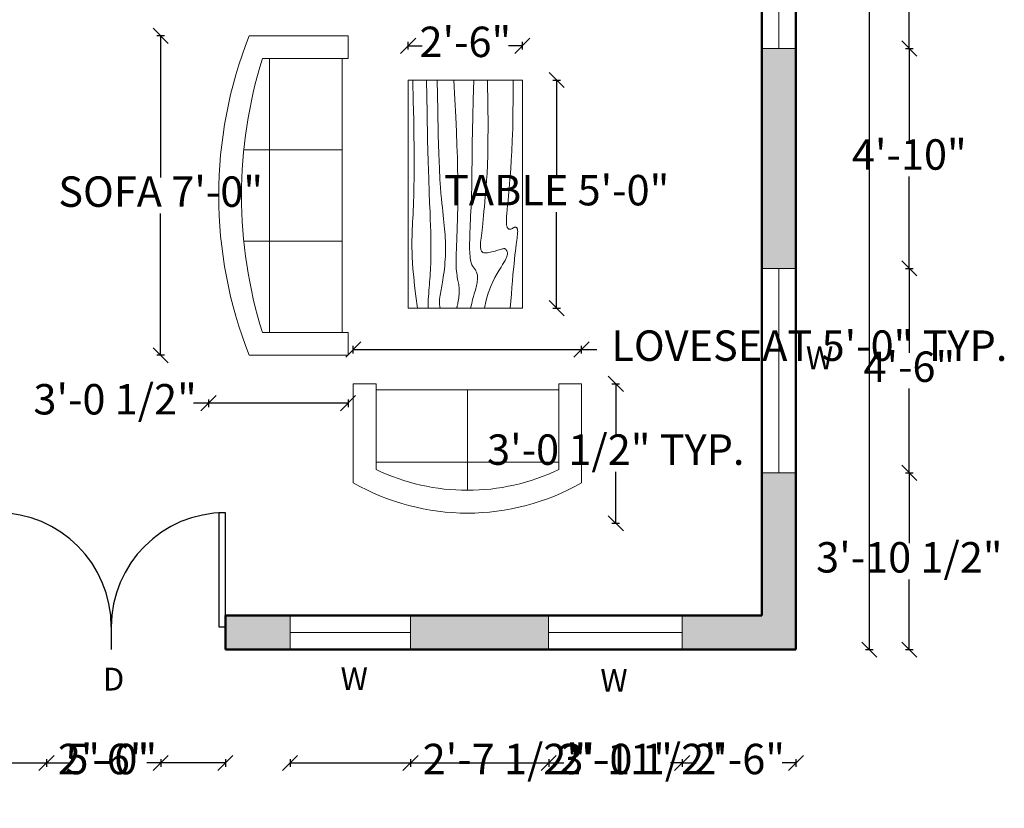
# Model space of a CAD drawing. Units: inches. Extents: x 2395 to 2921, y 528 to 1164.
# Tile 3 of 5: x 2662 to 2921, y 528 to 735. Entities that reach past the tile are written whole.
import ezdxf

# ---------------------------------------------------------------- set-up
doc = ezdxf.new("R2010")
doc.units = ezdxf.units.IN
for name, color, linetype, lineweight in [('A-ANNO-DIMS', 2, 'Continuous', 18), ('A-ANNO-TEXT', 7, 'Continuous', 18), ('A-DOOR', 3, 'Continuous', 25), ('A-FURN', 8, 'Continuous', 18), ('A-GLAZ', 4, 'Continuous', 18), ('A-WALL', 162, 'Continuous', 50), ('A-WALL-PATT', 162, 'Continuous', 13)]:
    doc.layers.add(name, color=color, linetype=linetype, lineweight=lineweight)
doc.styles.get("Standard").update_dxf_attribs({"font": 'arial.ttf'})
doc.dimstyles.new('ISO-25', dxfattribs={"dimtxt": 8, "dimasz": 4, "dimexe": 1, "dimexo": 1, "dimtad": 0, "dimtih": 1, "dimtoh": 1, "dimlunit": 3, "dimtxsty": 'Standard', "dimblk": 'OBLIQUE', "dimcen": 2.5, "dimadec": 0, "dimazin": 0, "dimtfac": 1, "dimtmove": 0, "dimatfit": 3, "dimfxl": 1, "dimfxlon": 1, "dimarcsym": 0})

# ---------------------------------------------------------------- blocks, each defined once
blk = doc.blocks.new('*U4')
for p, q in [((-30, 0), (-30, -6)), ((0, 0), (0, -6))]:
    blk.add_line(p, q)
blk.add_lwpolyline([(0, 0), (0, 30), (-1.75, 30), (-1.75, 0)], close=True)
blk.add_arc((0, 0), 30, 90, 180)
blk = doc.blocks.new('*U6')
for p, q in [((0, 0), (0, -6)), ((30, 0), (30, -6))]:
    blk.add_line(p, q)
blk.add_lwpolyline([(0, 0), (0, 30), (1.75, 30), (1.75, 0)], close=True)
blk.add_arc((0, 0), 30, 0, 90)
blk = doc.blocks.new('Sofa - Roundback 7 ft.')
for p, q in [((-12.00002, -32.4421), (-12.00003, -6.5971)), ((11.99997, -32.4421), (11.99998, -6.5971)), ((-36.000027, -34), (-36.000027, -11.4696)), ((35.99998, -34), (35.99998, -11.4696)), ((-35.999844, -13.3819), (35.9998, -13.3819)), ((-36.000027, -32.4421), (35.99998, -32.4421))]:
    blk.add_line(p, q)
for points in [[(-36.000027, -34), (-42.000027, -34), (-42.000027, -8)], [(41.99998, -8), (41.99998, -34), (35.99998, -34)]]:
    blk.add_lwpolyline(points)
for centre, radius, start, end in [((0, -114.25), 114.25, 68.43141, 111.5686), ((-0.00001, -127.1968), 121.1968, 72.72033, 107.2797)]:
    blk.add_arc(centre, radius, start, end)
blk = doc.blocks.new('Table - Rectangular Woodgrain 60 x 30 in.')
for p, q in [((0, 0), (0, -30)), ((60, 0), (0, 0)), ((60, -30), (60, 0)), ((0, -30), (60, -30))]:
    blk.add_line(p, q)
for points in [[(0, -2.4), (4.8155, -2.418), (9.0302, -2.4688), (12.709, -2.5477), (15.9167, -2.65), (18.7181, -2.7711), (21.1781, -2.9063), (23.3616, -3.0508), (25.3333, -3.2), (27.1477, -3.3495), (28.8172, -3.4958), (30.3437, -3.636), (31.7291, -3.7667), (32.9756, -3.8849), (34.0849, -3.9875), (35.059, -4.0714), (35.9, -4.1334), (36.6114, -4.1711), (37.2041, -4.1854), (37.6906, -4.1779), (38.0833, -4.15), (38.3948, -4.1034), (38.6375, -4.0396), (38.8239, -3.9602), (38.9666, -3.8667), (39.0764, -3.7608), (39.1573, -3.6448), (39.2116, -3.521), (39.2416, -3.3917), (39.2498, -3.2593), (39.2385, -3.1261), (39.21, -2.9944), (39.1666, -2.8667), (39.111, -2.7447), (39.0468, -2.6281), (38.978, -2.5163), (38.9083, -2.4083), (38.8418, -2.3035), (38.7823, -2.201), (38.7337, -2.1001), (38.7, -2), (38.6844, -1.9003), (38.6875, -1.8021), (38.7094, -1.707), (38.75, -1.6167), (38.8094, -1.5326), (38.8875, -1.4563), (38.9844, -1.3893), (39.1, -1.3333), (39.2351, -1.2896), (39.3937, -1.2583), (39.5804, -1.2396), (39.8, -1.2333), (40.057, -1.2396), (40.3562, -1.2583), (40.7023, -1.2896), (41.1, -1.3333), (41.5547, -1.3895), (42.0755, -1.4573), (42.6721, -1.5361), (43.3542, -1.625), (44.1316, -1.7233), (45.014, -1.8302), (46.0114, -1.9449), (47.1333, -2.0667), (48.3862, -2.1947), (49.7625, -2.3281), (51.2513, -2.4663), (52.8416, -2.6083), (54.5226, -2.7535), (56.2833, -2.9011), (58.1127, -3.0501), (60, -3.2)], [(0, -9.2), (6.5759, -9.0858), (11.9385, -9.0365), (16.2527, -9.0418), (19.6833, -9.0917), (22.3952, -9.1759), (24.5531, -9.2844), (26.322, -9.4069), (27.8666, -9.5333), (29.3241, -9.6553), (30.7203, -9.7719), (32.0532, -9.8837), (33.3208, -9.9917), (34.5213, -10.0965), (35.6526, -10.199), (36.7128, -10.2999), (37.7, -10.4), (38.6129, -10.4996), (39.4531, -10.5969), (40.223, -10.6895), (40.925, -10.775), (41.5613, -10.8512), (42.1344, -10.9156), (42.6465, -10.966), (43.1, -11), (43.4976, -11.0158), (43.8437, -11.0136), (44.143, -10.9942), (44.4, -10.9583), (44.6195, -10.9069), (44.8062, -10.8406), (44.9648, -10.7603), (45.1, -10.6667), (45.2155, -10.5598), (45.3114, -10.4365), (45.3871, -10.2929), (45.4416, -10.125), (45.4743, -9.929), (45.4844, -9.7011), (45.4709, -9.4371), (45.4333, -9.1333), (45.3716, -8.7883), (45.2896, -8.4104), (45.1919, -8.0107), (45.0833, -7.6), (44.9685, -7.1893), (44.8521, -6.7896), (44.7388, -6.4117), (44.6333, -6.0667), (44.54, -5.7628), (44.4614, -5.4979), (44.4001, -5.2675), (44.3583, -5.0667), (44.3384, -4.8909), (44.3427, -4.7354), (44.3736, -4.5956), (44.4333, -4.4667), (44.5236, -4.3453), (44.6427, -4.2333), (44.7884, -4.1339), (44.9583, -4.05), (45.1501, -3.9849), (45.3614, -3.9417), (45.59, -3.9234), (45.8333, -3.9333), (46.0915, -3.9749), (46.3734, -4.0531), (46.6906, -4.1736), (47.0542, -4.3417), (47.4756, -4.5629), (47.9661, -4.8427), (48.5372, -5.1866), (49.2, -5.6), (49.9676, -6.0844), (50.8594, -6.625), (51.8965, -7.2031), (53.1, -7.8), (54.491, -8.3969), (56.0906, -8.975), (57.9199, -9.5156), (60, -10)], [(0, -12.8), (5.1847, -12.9322), (9.6213, -13.0323), (13.3963, -13.1059), (16.5958, -13.1583), (19.3063, -13.1952), (21.614, -13.2219), (23.6054, -13.2439), (25.3666, -13.2667), (26.9728, -13.2947), (28.4531, -13.3281), (29.8256, -13.3663), (31.1083, -13.4083), (32.3191, -13.4535), (33.476, -13.501), (34.597, -13.5501), (35.7, -13.6), (36.7984, -13.6497), (37.8875, -13.6979), (38.9578, -13.743), (40, -13.7833), (41.0047, -13.8174), (41.9625, -13.8438), (42.864, -13.8607), (43.7, -13.8667), (44.4631, -13.8604), (45.1552, -13.8417), (45.7801, -13.8104), (46.3416, -13.7667), (46.8439, -13.7104), (47.2906, -13.6417), (47.6858, -13.5604), (48.0333, -13.4667), (48.3375, -13.3608), (48.6042, -13.2448), (48.8396, -13.121), (49.05, -12.9917), (49.2417, -12.8593), (49.4208, -12.7261), (49.5937, -12.5944), (49.7667, -12.4667), (49.9452, -12.3451), (50.1323, -12.2313), (50.3303, -12.1268), (50.5416, -12.0333), (50.7686, -11.9524), (51.0135, -11.8854), (51.2788, -11.8341), (51.5666, -11.8), (51.8785, -11.7843), (52.2116, -11.7865), (52.562, -11.8059), (52.926, -11.8417), (53.2998, -11.8931), (53.6795, -11.9594), (54.0614, -12.0397), (54.4416, -12.1333), (54.8223, -12.2401), (55.2293, -12.3625), (55.6942, -12.5037), (56.2489, -12.6667), (56.9251, -12.8547), (57.7545, -13.0708), (58.7689, -13.3182), (60, -13.6)], [(0, -18), (5.124, -17.7273), (9.6609, -17.5057), (13.6705, -17.3303), (17.2125, -17.1958), (20.3467, -17.0973), (23.1328, -17.0297), (25.6307, -16.9878), (27.9, -16.9667), (29.9928, -16.9617), (31.9302, -16.9703), (33.7254, -16.9907), (35.3917, -17.0208), (36.9423, -17.0588), (38.3906, -17.1026), (39.7499, -17.1503), (41.0333, -17.2), (42.2519, -17.2496), (43.4073, -17.2969), (44.4986, -17.3395), (45.525, -17.375), (46.4858, -17.4012), (47.3802, -17.4156), (48.2074, -17.416), (48.9667, -17.4), (49.6583, -17.3662), (50.2872, -17.3167), (50.8595, -17.2547), (51.3812, -17.1833), (51.8584, -17.1057), (52.2971, -17.025), (52.7034, -16.9443), (53.0833, -16.8667), (53.443, -16.7951), (53.789, -16.7313), (54.128, -16.6768), (54.4666, -16.6334), (54.8115, -16.6024), (55.1693, -16.5854), (55.5465, -16.5841), (55.95, -16.6), (56.3828, -16.6337), (56.8346, -16.6823), (57.2915, -16.7418), (57.7396, -16.8084), (58.165, -16.878), (58.5539, -16.9469), (58.8924, -17.0111), (59.1666, -17.0667), (59.3679, -17.1107), (59.5078, -17.1438), (59.6032, -17.1675), (59.6708, -17.1833), (59.7275, -17.193), (59.7901, -17.1979), (59.8753, -17.1998), (60, -17.2)], [(0, -22.4), (8.0098, -22.2501), (14.4094, -22.1011), (19.4168, -21.9535), (23.25, -21.8083), (26.1269, -21.6663), (28.2656, -21.5281), (29.884, -21.3947), (31.2, -21.2667), (32.3967, -21.1448), (33.5172, -21.0292), (34.5697, -20.9198), (35.5625, -20.8167), (36.5037, -20.7198), (37.4015, -20.6292), (38.2642, -20.5448), (39.1, -20.4667), (39.9164, -20.3951), (40.7187, -20.3313), (41.5117, -20.2768), (42.3, -20.2333), (43.0883, -20.2024), (43.8812, -20.1854), (44.6836, -20.1841), (45.5, -20.2), (46.3328, -20.234), (47.1747, -20.2844), (48.0163, -20.3488), (48.8479, -20.425), (49.66, -20.5106), (50.4429, -20.6031), (51.1872, -20.7004), (51.8833, -20.8), (52.5246, -20.8999), (53.1166, -20.9995), (53.6681, -21.0983), (54.1875, -21.1958), (54.6834, -21.2919), (55.1646, -21.3859), (55.6394, -21.4777), (56.1167, -21.5667), (56.6028, -21.6515), (57.0961, -21.7266), (57.5929, -21.7852), (58.0896, -21.8208), (58.5823, -21.8268), (59.0674, -21.7964), (59.5412, -21.723), (60, -21.6)], [(0, -25.2), (8.6355, -25.0504), (15.7026, -24.9031), (21.4049, -24.7606), (25.9458, -24.625), (29.529, -24.4988), (32.3578, -24.3844), (34.6359, -24.284), (36.5667, -24.2), (38.3213, -24.1341), (39.9417, -24.0854), (41.437, -24.0523), (42.8167, -24.0333), (44.0901, -24.0268), (45.2667, -24.0313), (46.3557, -24.0451), (47.3667, -24.0667), (48.309, -24.0947), (49.1928, -24.1287), (50.0284, -24.168), (50.826, -24.2125), (51.5959, -24.2617), (52.3483, -24.3151), (53.0935, -24.3725), (53.8417, -24.4334), (54.6009, -24.497), (55.3699, -24.561), (56.1454, -24.6226), (56.9239, -24.6792), (57.7021, -24.7279), (58.4764, -24.7662), (59.2435, -24.7911), (60, -24.8)], [(0, -28.8), (5.6867, -28.6681), (10.45, -28.5698), (14.407, -28.5012), (17.675, -28.4584), (20.3711, -28.4374), (22.6125, -28.4344), (24.5164, -28.4455), (26.2, -28.4667), (27.762, -28.4947), (29.2276, -28.5281), (30.6033, -28.5663), (31.8958, -28.6084), (33.1118, -28.6535), (34.2578, -28.7011), (35.3405, -28.7501), (36.3666, -28.8), (37.3443, -28.8497), (38.288, -28.8974), (39.2137, -28.9412), (40.1375, -28.9792), (41.0753, -29.0093), (42.0432, -29.0297), (43.0572, -29.0384), (44.1333, -29.0333), (45.2936, -29.0114), (46.5843, -28.9641), (48.0579, -28.8816), (49.7666, -28.7542), (51.7629, -28.5721), (54.0989, -28.3255), (56.8272, -28.0048), (60, -27.6)]]:
    blk.add_lwpolyline(points)
blk = doc.blocks.new('Sofa - Roundback Loveseat 5 ft.')
for p, q in [((0, -32.44198), (0, -5.99998)), ((-24, -33.99998), (-24, -11.46958)), ((24.00004, -33.99998), (24.00004, -11.46958)), ((-23.9998, -13.38178), (23.99986, -13.38178)), ((-24, -32.44198), (24.00004, -32.44198))]:
    blk.add_line(p, q)
for points in [[(-24, -33.99998), (-30, -33.99998), (-30, -7.99998)], [(30.00004, -7.99998), (30.00004, -33.99998), (24.00004, -33.99998)]]:
    blk.add_lwpolyline(points)
for centre, radius, start, end in [((0, -60.24998), 60.24998, 60.13715, 119.8628), ((0, -61.38438), 55.38444, 64.32083, 115.6792)]:
    blk.add_arc(centre, radius, start, end)
blk = doc.blocks.new('_Oblique')
at = {"color": 0, "linetype": 'ByBlock', "lineweight": -2}
blk.add_line((-0.5, -0.5), (0.5, 0.5), dxfattribs=at)
blk = doc.blocks.new('*D20')
at = {"layer": 'A-ANNO-DIMS', "color": 0, "lineweight": -2, "transparency": 16777216}
for p, q in [((2884.49, 1121.85), (2886.49, 1121.85)), ((2885.49, 1121.85), (2885.49, 850.56)), ((2885.49, 569.85), (2885.49, 841.14)), ((2884.49, 569.85), (2886.49, 569.85))]:
    blk.add_line(p, q, dxfattribs=at)
at = {"layer": 'Defpoints', "color": 0, "transparency": 16777216}
for p in [(2866.2, 1121.85), (2866.2, 569.85), (2885.49, 569.85)]:
    blk.add_point(p, dxfattribs=at)
at = {"layer": 'A-ANNO-DIMS', "color": 0, "lineweight": -2, "transparency": 16777216, "xscale": 4, "yscale": 4, "zscale": 4}
for p, rotation in [((2885.49, 1121.85), 90), ((2885.49, 569.85), 270)]:
    blk.add_blockref('_Oblique', p, dxfattribs=dict(at, rotation=rotation))
at = {"layer": 'A-ANNO-DIMS', "color": 0, "transparency": 16777216, "insert": (2885.49, 845.85), "char_height": 8, "attachment_point": 5}
blk.add_mtext("46'", dxfattribs=at)
blk = doc.blocks.new('*D28')
at = {"layer": 'A-ANNO-DIMS', "color": 0, "lineweight": -2, "transparency": 16777216}
for p, q in [((2749.83, 647.74), (2749.83, 649.74)), ((2809.83, 647.74), (2809.83, 649.74)), ((2749.83, 648.74), (2809.83, 648.74)), ((2809.83, 648.74), (2813.83, 648.74))]:
    blk.add_line(p, q, dxfattribs=at)
at = {"layer": 'Defpoints', "color": 0, "transparency": 16777216}
for p in [(2809.83, 648.74), (2749.83, 639.74), (2809.83, 639.74)]:
    blk.add_point(p, dxfattribs=at)
at = {"layer": 'A-ANNO-DIMS', "color": 0, "lineweight": -2, "transparency": 16777216, "xscale": 4, "yscale": 4, "zscale": 4, "rotation": 180}
blk.add_blockref('_Oblique', (2749.83, 648.74), dxfattribs=at)
at = {"layer": 'A-ANNO-DIMS', "color": 0, "lineweight": -2, "transparency": 16777216, "xscale": 4, "yscale": 4, "zscale": 4}
blk.add_blockref('_Oblique', (2809.83, 648.74), dxfattribs=at)
at = {"layer": 'A-ANNO-DIMS', "color": 0, "transparency": 16777216, "insert": (2869.72, 648.74), "char_height": 8, "attachment_point": 5}
blk.add_mtext('LOVESEAT 5\'-0" TYP.', dxfattribs=at)
blk = doc.blocks.new('*D29')
at = {"layer": 'A-ANNO-DIMS', "color": 0, "lineweight": -2, "transparency": 16777216}
for p, q in [((2817.83, 639.74), (2819.83, 639.74)), ((2818.83, 639.74), (2818.83, 626.17)), ((2818.83, 603.07), (2818.83, 616.64)), ((2817.83, 603.07), (2819.83, 603.07))]:
    blk.add_line(p, q, dxfattribs=at)
at = {"layer": 'Defpoints', "color": 0, "transparency": 16777216}
for p in [(2809.83, 639.74), (2809.83, 603.07), (2818.83, 603.07)]:
    blk.add_point(p, dxfattribs=at)
at = {"layer": 'A-ANNO-DIMS', "color": 0, "lineweight": -2, "transparency": 16777216, "xscale": 4, "yscale": 4, "zscale": 4}
for p, rotation in [((2818.83, 639.74), 90), ((2818.83, 603.07), 270)]:
    blk.add_blockref('_Oblique', p, dxfattribs=dict(at, rotation=rotation))
at = {"layer": 'A-ANNO-DIMS', "color": 0, "transparency": 16777216, "insert": (2818.83, 621.4), "char_height": 8, "attachment_point": 5}
blk.add_mtext('3\'-0 1/2" TYP.', dxfattribs=at)
blk = doc.blocks.new('*D32')
at = {"layer": 'A-ANNO-DIMS', "color": 0, "lineweight": -2, "transparency": 16777216}
for p, q in [((2700.18, 731.24), (2698.18, 731.24)), ((2699.18, 731.24), (2699.18, 694.01)), ((2699.18, 647.24), (2699.18, 684.48)), ((2700.18, 647.24), (2698.18, 647.24))]:
    blk.add_line(p, q, dxfattribs=at)
at = {"layer": 'Defpoints', "color": 0, "transparency": 16777216}
for p in [(2699.18, 731.24), (2711.78, 731.24), (2711.78, 647.24)]:
    blk.add_point(p, dxfattribs=at)
at = {"layer": 'A-ANNO-DIMS', "color": 0, "lineweight": -2, "transparency": 16777216, "xscale": 4, "yscale": 4, "zscale": 4}
for p, rotation in [((2699.18, 731.24), 90), ((2699.18, 647.24), 270)]:
    blk.add_blockref('_Oblique', p, dxfattribs=dict(at, rotation=rotation))
at = {"layer": 'A-ANNO-DIMS', "color": 0, "transparency": 16777216, "insert": (2699.18, 689.24), "char_height": 8, "attachment_point": 5}
blk.add_mtext('SOFA 7\'-0"', dxfattribs=at)
blk = doc.blocks.new('*D33')
at = {"layer": 'A-ANNO-DIMS', "color": 0, "lineweight": -2, "transparency": 16777216}
for p, q in [((2711.78, 634.64), (2707.78, 634.64)), ((2711.78, 635.64), (2711.78, 633.64)), ((2748.45, 634.64), (2711.78, 634.64)), ((2748.45, 635.64), (2748.45, 633.64))]:
    blk.add_line(p, q, dxfattribs=at)
at = {"layer": 'Defpoints', "color": 0, "transparency": 16777216}
for p in [(2711.78, 647.24), (2748.45, 647.24), (2711.78, 634.64)]:
    blk.add_point(p, dxfattribs=at)
at = {"layer": 'A-ANNO-DIMS', "color": 0, "lineweight": -2, "transparency": 16777216, "xscale": 4, "yscale": 4, "zscale": 4, "rotation": 180}
blk.add_blockref('_Oblique', (2711.78, 634.64), dxfattribs=at)
at = {"layer": 'A-ANNO-DIMS', "color": 0, "lineweight": -2, "transparency": 16777216, "xscale": 4, "yscale": 4, "zscale": 4}
blk.add_blockref('_Oblique', (2748.45, 634.64), dxfattribs=at)
at = {"layer": 'A-ANNO-DIMS', "color": 0, "transparency": 16777216, "insert": (2687.21, 634.64), "char_height": 8, "attachment_point": 5}
blk.add_mtext('3\'-0 1/2"', dxfattribs=at)
blk = doc.blocks.new('*D34')
at = {"layer": 'A-ANNO-DIMS', "color": 0, "lineweight": -2, "transparency": 16777216}
for p, q in [((2802.28, 719.62), (2804.28, 719.62)), ((2803.28, 719.62), (2803.28, 694.33)), ((2803.28, 659.62), (2803.28, 684.91)), ((2802.28, 659.62), (2804.28, 659.62))]:
    blk.add_line(p, q, dxfattribs=at)
at = {"layer": 'Defpoints', "color": 0, "transparency": 16777216}
for p in [(2794.28, 719.62), (2794.28, 659.62), (2803.28, 659.62)]:
    blk.add_point(p, dxfattribs=at)
at = {"layer": 'A-ANNO-DIMS', "color": 0, "lineweight": -2, "transparency": 16777216, "xscale": 4, "yscale": 4, "zscale": 4}
for p, rotation in [((2803.28, 719.62), 90), ((2803.28, 659.62), 270)]:
    blk.add_blockref('_Oblique', p, dxfattribs=dict(at, rotation=rotation))
at = {"layer": 'A-ANNO-DIMS', "color": 0, "transparency": 16777216, "insert": (2803.28, 689.62), "char_height": 8, "attachment_point": 5}
blk.add_mtext('TABLE 5\'-0"', dxfattribs=at)
blk = doc.blocks.new('*D35')
at = {"layer": 'A-ANNO-DIMS', "color": 0, "lineweight": -2, "transparency": 16777216}
for p, q in [((2764.28, 727.62), (2764.28, 729.62)), ((2764.28, 728.62), (2767.95, 728.62)), ((2794.28, 728.62), (2790.6, 728.62)), ((2794.28, 727.62), (2794.28, 729.62))]:
    blk.add_line(p, q, dxfattribs=at)
at = {"layer": 'Defpoints', "color": 0, "transparency": 16777216}
for p in [(2794.28, 728.62), (2764.28, 719.62), (2794.28, 719.62)]:
    blk.add_point(p, dxfattribs=at)
at = {"layer": 'A-ANNO-DIMS', "color": 0, "lineweight": -2, "transparency": 16777216, "xscale": 4, "yscale": 4, "zscale": 4, "rotation": 180}
blk.add_blockref('_Oblique', (2764.28, 728.62), dxfattribs=at)
at = {"layer": 'A-ANNO-DIMS', "color": 0, "lineweight": -2, "transparency": 16777216, "xscale": 4, "yscale": 4, "zscale": 4}
blk.add_blockref('_Oblique', (2794.28, 728.62), dxfattribs=at)
at = {"layer": 'A-ANNO-DIMS', "color": 0, "transparency": 16777216, "insert": (2779.28, 728.62), "char_height": 8, "attachment_point": 5}
blk.add_mtext('2\'-6"', dxfattribs=at)
blk = doc.blocks.new('*D45')
at = {"layer": 'A-ANNO-DIMS', "color": 0, "lineweight": -2, "transparency": 16777216}
for p, q in [((2656.2, 541.05), (2656.2, 539.05)), ((2716.2, 541.05), (2716.2, 539.05)), ((2656.2, 540.05), (2674.94, 540.05)), ((2716.2, 540.05), (2697.46, 540.05))]:
    blk.add_line(p, q, dxfattribs=at)
at = {"layer": 'Defpoints', "color": 0, "transparency": 16777216}
for p in [(2656.2, 569.85), (2716.2, 569.85), (2716.2, 540.05)]:
    blk.add_point(p, dxfattribs=at)
at = {"layer": 'A-ANNO-DIMS', "color": 0, "lineweight": -2, "transparency": 16777216, "xscale": 4, "yscale": 4, "zscale": 4, "rotation": 180}
blk.add_blockref('_Oblique', (2656.2, 540.05), dxfattribs=at)
at = {"layer": 'A-ANNO-DIMS', "color": 0, "lineweight": -2, "transparency": 16777216, "xscale": 4, "yscale": 4, "zscale": 4}
blk.add_blockref('_Oblique', (2716.2, 540.05), dxfattribs=at)
at = {"layer": 'A-ANNO-DIMS', "color": 0, "transparency": 16777216, "insert": (2686.2, 540.05), "char_height": 8, "attachment_point": 5}
blk.add_mtext('5\'-0"', dxfattribs=at)
blk = doc.blocks.new('*D46')
at = {"layer": 'A-ANNO-DIMS', "color": 0, "lineweight": -2, "transparency": 16777216}
for p, q in [((2733.2, 541.05), (2733.2, 539.05)), ((2764.89, 541.05), (2764.89, 539.05)), ((2733.2, 540.05), (2764.89, 540.05)), ((2764.89, 540.05), (2768.89, 540.05))]:
    blk.add_line(p, q, dxfattribs=at)
at = {"layer": 'Defpoints', "color": 0, "transparency": 16777216}
for p in [(2733.2, 569.85), (2764.89, 569.85), (2764.89, 540.05)]:
    blk.add_point(p, dxfattribs=at)
at = {"layer": 'A-ANNO-DIMS', "color": 0, "lineweight": -2, "transparency": 16777216, "xscale": 4, "yscale": 4, "zscale": 4, "rotation": 180}
blk.add_blockref('_Oblique', (2733.2, 540.05), dxfattribs=at)
at = {"layer": 'A-ANNO-DIMS', "color": 0, "lineweight": -2, "transparency": 16777216, "xscale": 4, "yscale": 4, "zscale": 4}
blk.add_blockref('_Oblique', (2764.89, 540.05), dxfattribs=at)
at = {"layer": 'A-ANNO-DIMS', "color": 0, "transparency": 16777216, "insert": (2789.54, 540.05), "char_height": 8, "attachment_point": 5}
blk.add_mtext('2\'-7 1/2"', dxfattribs=at)
blk = doc.blocks.new('*D47')
at = {"layer": 'A-ANNO-DIMS', "color": 0, "lineweight": -2, "transparency": 16777216}
for p, q in [((2764.89, 541.05), (2764.89, 539.05)), ((2801.19, 541.05), (2801.19, 539.05)), ((2764.89, 540.05), (2801.19, 540.05)), ((2801.19, 540.05), (2805.19, 540.05))]:
    blk.add_line(p, q, dxfattribs=at)
at = {"layer": 'Defpoints', "color": 0, "transparency": 16777216}
for p in [(2764.89, 569.85), (2801.19, 569.85), (2801.19, 540.05)]:
    blk.add_point(p, dxfattribs=at)
at = {"layer": 'A-ANNO-DIMS', "color": 0, "lineweight": -2, "transparency": 16777216, "xscale": 4, "yscale": 4, "zscale": 4, "rotation": 180}
blk.add_blockref('_Oblique', (2764.89, 540.05), dxfattribs=at)
at = {"layer": 'A-ANNO-DIMS', "color": 0, "lineweight": -2, "transparency": 16777216, "xscale": 4, "yscale": 4, "zscale": 4}
blk.add_blockref('_Oblique', (2801.19, 540.05), dxfattribs=at)
at = {"layer": 'A-ANNO-DIMS', "color": 0, "transparency": 16777216, "insert": (2825.76, 540.05), "char_height": 8, "attachment_point": 5}
blk.add_mtext('3\'-0 1/2"', dxfattribs=at)
blk = doc.blocks.new('*D48')
at = {"layer": 'A-ANNO-DIMS', "color": 0, "lineweight": -2, "transparency": 16777216}
for p, q in [((2801.19, 541.05), (2801.19, 539.05)), ((2836.31, 541.05), (2836.31, 539.05)), ((2801.19, 540.05), (2804.32, 540.05)), ((2836.31, 540.05), (2833.19, 540.05))]:
    blk.add_line(p, q, dxfattribs=at)
at = {"layer": 'Defpoints', "color": 0, "transparency": 16777216}
for p in [(2801.19, 569.85), (2836.31, 569.85), (2836.31, 540.05)]:
    blk.add_point(p, dxfattribs=at)
at = {"layer": 'A-ANNO-DIMS', "color": 0, "lineweight": -2, "transparency": 16777216, "xscale": 4, "yscale": 4, "zscale": 4, "rotation": 180}
blk.add_blockref('_Oblique', (2801.19, 540.05), dxfattribs=at)
at = {"layer": 'A-ANNO-DIMS', "color": 0, "lineweight": -2, "transparency": 16777216, "xscale": 4, "yscale": 4, "zscale": 4}
blk.add_blockref('_Oblique', (2836.31, 540.05), dxfattribs=at)
at = {"layer": 'A-ANNO-DIMS', "color": 0, "transparency": 16777216, "insert": (2818.75, 540.05), "char_height": 8, "attachment_point": 5}
blk.add_mtext('2\'-11"', dxfattribs=at)
blk = doc.blocks.new('*D49')
at = {"layer": 'A-ANNO-DIMS', "color": 0, "lineweight": -2, "transparency": 16777216}
for p, q in [((2836.31, 541.05), (2836.31, 539.05)), ((2866.2, 541.05), (2866.2, 539.05)), ((2836.31, 540.05), (2839.93, 540.05)), ((2866.2, 540.05), (2862.58, 540.05))]:
    blk.add_line(p, q, dxfattribs=at)
at = {"layer": 'Defpoints', "color": 0, "transparency": 16777216}
for p in [(2836.31, 569.85), (2866.2, 569.85), (2866.2, 540.05)]:
    blk.add_point(p, dxfattribs=at)
at = {"layer": 'A-ANNO-DIMS', "color": 0, "lineweight": -2, "transparency": 16777216, "xscale": 4, "yscale": 4, "zscale": 4, "rotation": 180}
blk.add_blockref('_Oblique', (2836.31, 540.05), dxfattribs=at)
at = {"layer": 'A-ANNO-DIMS', "color": 0, "lineweight": -2, "transparency": 16777216, "xscale": 4, "yscale": 4, "zscale": 4}
blk.add_blockref('_Oblique', (2866.2, 540.05), dxfattribs=at)
at = {"layer": 'A-ANNO-DIMS', "color": 0, "transparency": 16777216, "insert": (2851.26, 540.05), "char_height": 8, "attachment_point": 5}
blk.add_mtext('2\'-6"', dxfattribs=at)
blk = doc.blocks.new('*D62')
at = {"layer": 'A-ANNO-DIMS', "color": 0, "lineweight": -2, "transparency": 16777216}
for p, q in [((2895, 616.31), (2897, 616.31)), ((2896, 616.31), (2896, 597.84)), ((2896, 569.85), (2896, 588.32)), ((2895, 569.85), (2897, 569.85))]:
    blk.add_line(p, q, dxfattribs=at)
at = {"layer": 'Defpoints', "color": 0, "transparency": 16777216}
for p in [(2866.2, 616.31), (2896, 616.31), (2866.2, 569.85)]:
    blk.add_point(p, dxfattribs=at)
at = {"layer": 'A-ANNO-DIMS', "color": 0, "lineweight": -2, "transparency": 16777216, "xscale": 4, "yscale": 4, "zscale": 4}
for p, rotation in [((2896, 616.31), 90), ((2896, 569.85), 270)]:
    blk.add_blockref('_Oblique', p, dxfattribs=dict(at, rotation=rotation))
at = {"layer": 'A-ANNO-DIMS', "color": 0, "transparency": 16777216, "insert": (2896, 593.08), "char_height": 8, "attachment_point": 5}
blk.add_mtext('3\'-10 1/2"', dxfattribs=at)
blk = doc.blocks.new('*D63')
at = {"layer": 'A-ANNO-DIMS', "color": 0, "lineweight": -2, "transparency": 16777216}
for p, q in [((2895, 670.09), (2897, 670.09)), ((2896, 670.09), (2896, 647.91)), ((2896, 616.31), (2896, 638.49)), ((2895, 616.31), (2897, 616.31))]:
    blk.add_line(p, q, dxfattribs=at)
at = {"layer": 'Defpoints', "color": 0, "transparency": 16777216}
for p in [(2866.2, 670.09), (2896, 670.09), (2866.2, 616.31)]:
    blk.add_point(p, dxfattribs=at)
at = {"layer": 'A-ANNO-DIMS', "color": 0, "lineweight": -2, "transparency": 16777216, "xscale": 4, "yscale": 4, "zscale": 4}
for p, rotation in [((2896, 670.09), 90), ((2896, 616.31), 270)]:
    blk.add_blockref('_Oblique', p, dxfattribs=dict(at, rotation=rotation))
at = {"layer": 'A-ANNO-DIMS', "color": 0, "transparency": 16777216, "insert": (2896, 643.2), "char_height": 8, "attachment_point": 5}
blk.add_mtext('4\'-6"', dxfattribs=at)
blk = doc.blocks.new('*D64')
at = {"layer": 'A-ANNO-DIMS', "color": 0, "lineweight": -2, "transparency": 16777216}
for p, q in [((2895, 727.91), (2897, 727.91)), ((2896, 727.91), (2896, 703.71)), ((2896, 670.09), (2896, 694.29)), ((2895, 670.09), (2897, 670.09))]:
    blk.add_line(p, q, dxfattribs=at)
at = {"layer": 'Defpoints', "color": 0, "transparency": 16777216}
for p in [(2866.2, 727.91), (2896, 727.91), (2866.2, 670.09)]:
    blk.add_point(p, dxfattribs=at)
at = {"layer": 'A-ANNO-DIMS', "color": 0, "lineweight": -2, "transparency": 16777216, "xscale": 4, "yscale": 4, "zscale": 4}
for p, rotation in [((2896, 727.91), 90), ((2896, 670.09), 270)]:
    blk.add_blockref('_Oblique', p, dxfattribs=dict(at, rotation=rotation))
at = {"layer": 'A-ANNO-DIMS', "color": 0, "transparency": 16777216, "insert": (2896, 699), "char_height": 8, "attachment_point": 5}
blk.add_mtext('4\'-10"', dxfattribs=at)
blk = doc.blocks.new('*D65')
at = {"layer": 'A-ANNO-DIMS', "color": 0, "lineweight": -2, "transparency": 16777216}
for p, q in [((2895, 777.1), (2897, 777.1)), ((2896, 777.1), (2896, 757.14)), ((2896, 727.91), (2896, 747.86)), ((2895, 727.91), (2897, 727.91))]:
    blk.add_line(p, q, dxfattribs=at)
at = {"layer": 'Defpoints', "color": 0, "transparency": 16777216}
for p in [(2866.2, 777.1), (2896, 777.1), (2866.2, 727.91)]:
    blk.add_point(p, dxfattribs=at)
at = {"layer": 'A-ANNO-DIMS', "color": 0, "lineweight": -2, "transparency": 16777216, "xscale": 4, "yscale": 4, "zscale": 4}
for p, rotation in [((2896, 777.1), 90), ((2896, 727.91), 270)]:
    blk.add_blockref('_Oblique', p, dxfattribs=dict(at, rotation=rotation))
at = {"layer": 'A-ANNO-DIMS', "color": 0, "transparency": 16777216, "insert": (2896, 752.5), "char_height": 8, "attachment_point": 5}
blk.add_mtext('4\'-1"', dxfattribs=at)
blk = doc.blocks.new('*D73')
at = {"layer": 'A-ANNO-DIMS', "color": 0, "lineweight": -2, "transparency": 16777216}
for p, q in [((2669.2, 541.05), (2669.2, 539.05)), ((2699.2, 541.05), (2699.2, 539.05)), ((2669.2, 540.05), (2672.87, 540.05)), ((2699.2, 540.05), (2695.53, 540.05))]:
    blk.add_line(p, q, dxfattribs=at)
at = {"layer": 'Defpoints', "color": 0, "transparency": 16777216}
for p in [(2669.2, 988.35), (2699.2, 988.35), (2699.2, 540.05)]:
    blk.add_point(p, dxfattribs=at)
at = {"layer": 'A-ANNO-DIMS', "color": 0, "lineweight": -2, "transparency": 16777216, "xscale": 4, "yscale": 4, "zscale": 4, "rotation": 180}
blk.add_blockref('_Oblique', (2669.2, 540.05), dxfattribs=at)
at = {"layer": 'A-ANNO-DIMS', "color": 0, "lineweight": -2, "transparency": 16777216, "xscale": 4, "yscale": 4, "zscale": 4}
blk.add_blockref('_Oblique', (2699.2, 540.05), dxfattribs=at)
at = {"layer": 'A-ANNO-DIMS', "color": 0, "transparency": 16777216, "insert": (2684.2, 540.05), "char_height": 8, "attachment_point": 5}
blk.add_mtext('2\'-6"', dxfattribs=at)

msp = doc.modelspace()

# ---------------------------------------------------------------- hatches: boundary and pattern name
at = {"layer": 'A-WALL-PATT'}
h = msp.add_hatch(color=256, dxfattribs=at)
h.dxf.hatch_style = 1
h.paths.add_polyline_path([(2627.2, 1121.853), (2446.2, 1121.853), (2446.2, 1054.648), (2455.2, 1054.648), (2455.2, 1112.853), (2606.2, 1112.853), (2606.2, 1022.853), (2610.7, 1022.853), (2610.7, 1112.853), (2627.2, 1112.853)])
h.paths.add_polyline_path([(2685.7, 1121.853), (2648.2, 1121.853), (2648.2, 1112.853), (2664.7, 1112.853), (2664.7, 992.853), (2606.2, 992.853), (2606.2, 962.853), (2610.7, 962.853), (2610.7, 988.353), (2669.2, 988.353), (2669.2, 994.353), (2669.2, 1024.353), (2669.2, 1112.853), (2685.7, 1112.853)])
h.paths.add_polyline_path([(2866.2, 1121.853), (2706.7, 1121.853), (2706.7, 1112.853), (2723.2, 1112.853), (2723.2, 992.853), (2699.2, 992.853), (2699.2, 988.353), (2723.2, 988.353), (2723.2, 962.853), (2727.7, 962.853), (2727.7, 1112.853), (2857.2, 1112.853), (2857.2, 1049.508), (2866.2, 1049.508)])
h.paths.add_polyline_path([(2866.2, 985.129), (2857.2, 985.129), (2857.2, 926.853), (2723.2, 926.853), (2723.2, 922.353), (2729.2, 922.353), (2765.2, 922.353), (2857.2, 922.353), (2857.2, 894.873), (2866.2, 894.873)])
h.paths.add_polyline_path([(2455.2, 997.652), (2446.2, 997.652), (2446.2, 909.181), (2455.2, 908.938), (2455.2, 922.353), (2610.7, 922.353), (2610.7, 926.853), (2455.2, 926.853)])
h.paths.add_polyline_path([(2455.2, 838.353), (2610.7, 838.353), (2610.7, 842.853), (2455.2, 842.853), (2455.2, 856.236), (2446.2, 856.236), (2446.2, 815.427), (2455.2, 815.427)])
h.paths.add_polyline_path([(2455.2, 772.706), (2446.2, 772.706), (2446.2, 569.853), (2505.031, 569.853), (2505.031, 578.853), (2455.2, 578.853), (2455.2, 734.853), (2570.2, 734.853), (2570.2, 739.353), (2568.7, 739.353), (2568.7, 806.353), (2564.2, 806.353), (2564.2, 739.353), (2455.2, 739.353)])
h.paths.add_polyline_path([(2656.2, 578.853), (2610.7, 578.853), (2610.7, 739.353), (2606.2, 739.353), (2606.2, 578.853), (2565.031, 578.853), (2565.031, 569.853), (2656.2, 569.853)])
h.paths.add_polyline_path([(2733.198, 578.853), (2716.2, 578.853), (2716.2, 569.853), (2733.198, 569.853)])
h.paths.add_polyline_path([(2801.188, 578.853), (2764.893, 578.853), (2764.893, 569.853), (2801.188, 569.853)])
h.paths.add_polyline_path([(2866.2, 616.306), (2857.2, 616.306), (2857.2, 578.853), (2836.314, 578.853), (2836.314, 569.853), (2866.2, 569.853)])
h.paths.add_polyline_path([(2866.2, 727.906), (2857.2, 727.906), (2857.2, 670.095), (2866.2, 670.095)])
h.paths.add_polyline_path([(2866.2, 831.149), (2857.2, 831.149), (2857.2, 795.353), (2727.7, 795.353), (2727.7, 886.353), (2723.2, 886.353), (2723.2, 790.853), (2857.2, 790.853), (2857.2, 777.101), (2866.2, 777.101)])

# ---------------------------------------------------------------- linework, layer by layer
at = {"layer": 'A-GLAZ'}
for p, q in [((2861.7, 727.906), (2861.7, 777.101)), ((2857.2, 727.906), (2866.2, 727.906)), ((2857.2, 670.095), (2866.2, 670.095)), ((2861.7, 616.306), (2861.7, 670.095)), ((2857.2, 616.306), (2866.2, 616.306)), ((2733.198, 578.853), (2733.198, 569.853)), ((2764.893, 578.853), (2764.893, 569.853)), ((2801.188, 578.853), (2801.188, 569.853)), ((2836.314, 578.853), (2836.314, 569.853)), ((2733.198, 574.353), (2764.893, 574.353)), ((2801.188, 574.353), (2836.314, 574.353))]:
    msp.add_line(p, q, dxfattribs=at)
at = {"layer": 'A-WALL'}
for p, q in [((2866.2, 569.853), (2866.2, 1121.853)), ((2857.2, 578.853), (2857.2, 790.853)), ((2716.2, 578.853), (2716.2, 569.853)), ((2716.2, 578.853), (2857.2, 578.853)), ((2716.2, 569.853), (2866.2, 569.853))]:
    msp.add_line(p, q, dxfattribs=at)

# ---------------------------------------------------------------- block references
at = {"layer": 'A-DOOR'}
for name, p in [('*U6', (2656.2, 575.853)), ('*U4', (2716.2, 575.853))]:
    msp.add_blockref(name, p, dxfattribs=at)
at = {"layer": 'A-FURN'}
for name, p, rotation in [('Sofa - Roundback 7 ft.', (2714.45, 689.242), 90), ('Table - Rectangular Woodgrain 60 x 30 in.', (2794.277, 719.623), 270)]:
    msp.add_blockref(name, p, dxfattribs=dict(at, rotation=rotation))
at = {"layer": 'A-FURN', "xscale": -1, "rotation": 180}
msp.add_blockref('Sofa - Roundback Loveseat 5 ft.', (2779.83, 605.738), dxfattribs=at)

# ---------------------------------------------------------------- texts
at = {"layer": 'A-ANNO-TEXT', "char_height": 6, "attachment_point": 1}
for s, insert in [('\\pxqc;W', (2866.2, 649.577)), ('\\pxqc;D', (2680.59, 565.087)), ('\\pxqc;W', (2743.858, 565.191)), ('\\pxqc;W', (2812.149, 564.782))]:
    msp.add_mtext_dynamic_manual_height_columns(s, width=12.42697, gutter_width=12.5, heights=[0], dxfattribs=dict(at, insert=insert))

# ---------------------------------------------------------------- dimensions: what is measured, and where the dimension line sits
at = {"layer": 'A-ANNO-DIMS'}
for base, p1, p2, angle, override, picture, middle in [((2885.489, 569.853), (2866.2, 1121.853), (2866.2, 569.853), 90, {"dimclrd": 0, "dimclre": 0, "dimclrt": 0}, '*D20', (2885.489, 845.853)), ((2896, 777.101), (2866.2, 727.906), (2866.2, 777.101), 90, {"dimdec": 1, "dimlfac": 1, "dimrnd": 0, "dimzin": 1, "dimdsep": 46, "dimlunit": 4, "dimfrac": 2}, '*D65', (2896, 752.503)), ((2896, 727.906), (2866.2, 670.095), (2866.2, 727.906), 90, {"dimdec": 1, "dimlfac": 1, "dimrnd": 0, "dimzin": 1, "dimdsep": 46, "dimlunit": 4, "dimfrac": 2}, '*D64', (2896, 699)), ((2896, 670.095), (2866.2, 616.306), (2866.2, 670.095), 90, {"dimdec": 1, "dimlfac": 1, "dimrnd": 0, "dimzin": 1, "dimdsep": 46, "dimlunit": 4, "dimfrac": 2}, '*D63', (2896, 643.201)), ((2711.783, 634.642), (2748.45, 647.242), (2711.783, 647.242), 180, {"dimdec": 1, "dimlfac": 1, "dimrnd": 0, "dimzin": 1, "dimdsep": 46, "dimlunit": 4, "dimfrac": 2}, '*D33', (2687.207, 634.642)), ((2896, 616.306), (2866.2, 569.853), (2866.2, 616.306), 90, {"dimdec": 1, "dimlfac": 1, "dimrnd": 0, "dimzin": 1, "dimdsep": 46, "dimlunit": 4, "dimfrac": 2}, '*D62', (2896, 593.08))]:
    dim = msp.add_linear_dim(base=base, p1=p1, p2=p2, angle=angle, dimstyle='ISO-25', override=override, dxfattribs=at)
    dim.commit()
    dim.dimension.update_dxf_attribs({"geometry": picture, "text_midpoint": middle})
for base, p1, p2, picture, middle in [((2699.2, 540.053), (2669.2, 988.353), (2699.2, 988.353), '*D73', (2684.2, 540.053)), ((2794.277, 728.623), (2764.277, 719.623), (2794.277, 719.623), '*D35', (2779.277, 728.623)), ((2716.2, 540.053), (2656.2, 569.853), (2716.2, 569.853), '*D45', (2686.2, 540.053)), ((2764.893, 540.053), (2733.198, 569.853), (2764.893, 569.853), '*D46', (2789.54, 540.053)), ((2801.188, 540.053), (2764.893, 569.853), (2801.188, 569.853), '*D47', (2825.764, 540.053)), ((2836.314, 540.053), (2801.188, 569.853), (2836.314, 569.853), '*D48', (2818.751, 540.053)), ((2866.2, 540.053), (2836.314, 569.853), (2866.2, 569.853), '*D49', (2851.257, 540.053))]:
    dim = msp.add_linear_dim(base=base, p1=p1, p2=p2, dimstyle='ISO-25', override={"dimdec": 1, "dimlfac": 1, "dimrnd": 0, "dimzin": 1, "dimdsep": 46, "dimlunit": 4, "dimfrac": 2}, dxfattribs=at)
    dim.commit()
    dim.dimension.update_dxf_attribs({"geometry": picture, "text_midpoint": middle})
for base, p1, p2, angle, text, picture, middle in [((2699.183, 731.242), (2711.783, 647.242), (2711.783, 731.242), 90, 'SOFA <>', '*D32', (2699.183, 689.242)), ((2803.277, 659.623), (2794.277, 719.623), (2794.277, 659.623), 270, 'TABLE <>', '*D34', (2803.277, 689.623)), ((2818.83, 603.071), (2809.83, 639.738), (2809.83, 603.071), 270, '<> TYP.', '*D29', (2818.83, 621.405))]:
    dim = msp.add_linear_dim(base=base, p1=p1, p2=p2, angle=angle, text=text, dimstyle='ISO-25', override={"dimdec": 1, "dimlfac": 1, "dimrnd": 0, "dimzin": 1, "dimdsep": 46, "dimlunit": 4, "dimfrac": 2}, dxfattribs=at)
    dim.commit()
    dim.dimension.update_dxf_attribs({"geometry": picture, "text_midpoint": middle})
dim = msp.add_linear_dim(base=(2809.83, 648.738), p1=(2749.83, 639.738), p2=(2809.83, 639.738), text='LOVESEAT <> TYP.', dimstyle='ISO-25', override={"dimdec": 1, "dimlfac": 1, "dimrnd": 0, "dimzin": 1, "dimdsep": 46, "dimlunit": 4, "dimfrac": 2}, dxfattribs=at)
dim.commit()
dim.dimension.update_dxf_attribs({"geometry": '*D28', "text_midpoint": (2869.716, 648.738)})

doc.saveas('drawing.dxf')
